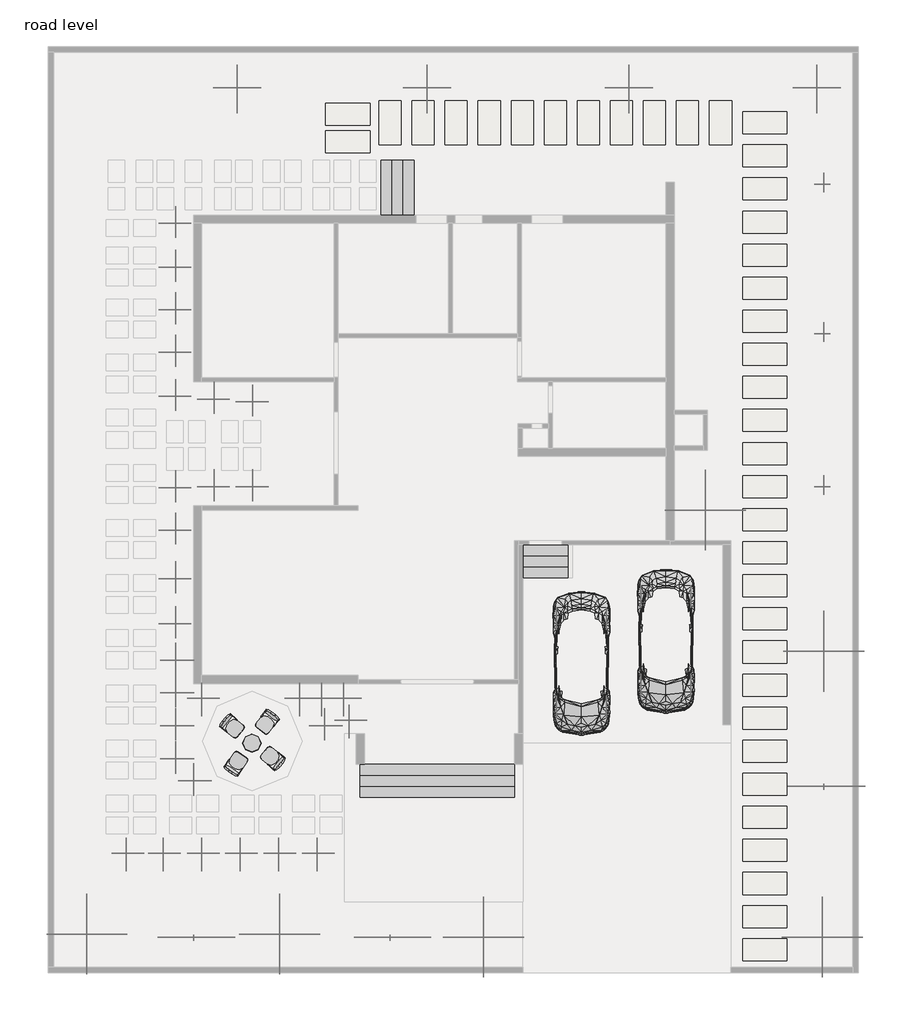
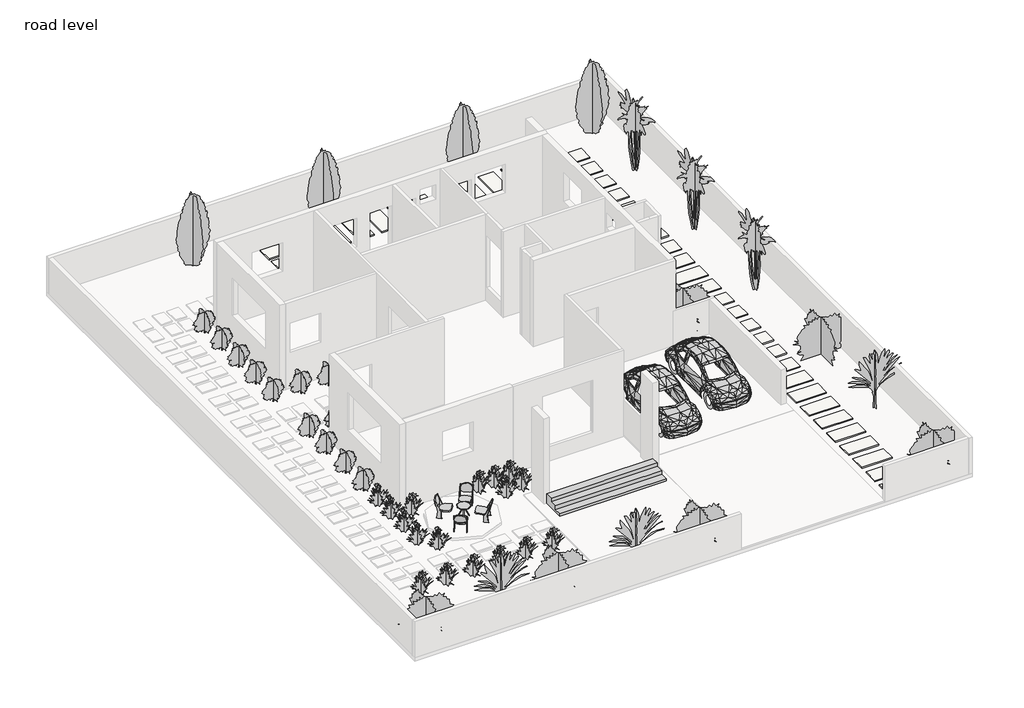
# One storey, part 3 of 3: 46 geographic elements, 8 furniture elements, 2 proxies, 1 slab.
"""IFC4 building model written with IfcOpenShell, lengths in millimetres."""

from ifc_helpers import new_model, si_unit, origin, origin_with_axes, place, context, project, spatial, polyline, outline, extrude, transform, mapped, element, save
from components import rpc_beetle_rpc_beetle_31f8b51e, casework_1_casework_1_95f3130b, casework_2_casework_2_cc4890fd, casework_3_casework_3_0f97de66, furniture_eb3a3c23, furniture_9d41381f, rpc_plant_tropical_55f6ff97, rpc_plant_tropical_jungle_flame_3_9c4808c2, rpc_shrub_d2795376, rpc_tree_deciduous_japanese_maple_10_8b15208c, rpc_tree_tropical_golden_malay_palm_10_e9996539, rpc_tree_tropical_japanese_fiber_banana_8_86d3d22d

model = new_model("IFC4")

# Units and contexts
model_context = context("Model", 3, world=origin())
ifc_project = project(units=[si_unit("LENGTHUNIT", "METRE", prefix="MILLI")], contexts=[model_context])

# Site, building, storey
site = spatial("IfcSite", under=ifc_project)
building = spatial("IfcBuilding", under=site)
storey = spatial("IfcBuildingStorey", under=building, Name="road level", Elevation=0.0)

# Proxies
placement = place(None, origin())
rpc_beetle_rpc_beetle_shape = rpc_beetle_rpc_beetle_31f8b51e(model_context)
element("IfcBuildingElementProxy", 1, Name="RPC Beetle : RPC Beetle", ObjectType="RPC Beetle : RPC Beetle", at=placement, inside=storey, context=model_context, shape_type="MappedRepresentation", body=[
    mapped(rpc_beetle_rpc_beetle_shape, transform((-917.8719122, 43.2168074, 50.8), x_axis=(-1.0, 0.0, 0.0), y_axis=(0.0, -1.0, 0.0), z_axis=(0.0, 0.0, 1.0))),
])
element("IfcBuildingElementProxy", 2, Name="RPC Beetle : RPC Beetle", ObjectType="RPC Beetle : RPC Beetle", at=placement, inside=storey, context=model_context, shape_type="MappedRepresentation", body=[
    mapped(rpc_beetle_rpc_beetle_shape, transform((-3254.6719122, -566.3831926, 50.8), x_axis=(-1.0, 0.0, 0.0), y_axis=(0.0, -1.0, 0.0), z_axis=(0.0, 0.0, 1.0))),
])

# Furniture
casework_1_casework_1_shape = casework_1_casework_1_95f3130b(model_context)
element("IfcFurniture", 3, ObjectType="Casework 1 : Casework 1", at=placement, inside=storey, context=model_context, shape_type="MappedRepresentation", body=[
    mapped(casework_1_casework_1_shape, transform((0.0, -844.55, -1397.3720703), x_axis=(1.0, 0.0, 0.0), y_axis=(0.0, 1.0, 0.0), z_axis=(0.0, 0.0, 1.0))),
])
casework_2_casework_2_shape = casework_2_casework_2_cc4890fd(model_context)
element("IfcFurniture", 4, ObjectType="Casework 2 : Casework 2", at=placement, inside=storey, context=model_context, shape_type="MappedRepresentation", body=[
    mapped(casework_2_casework_2_shape, transform((-2752.725, 0.0, -762.0), x_axis=(1.0, 0.0, 0.0), y_axis=(0.0, 1.0, 0.0), z_axis=(0.0, 0.0, 1.0))),
])
casework_3_casework_3_shape = casework_3_casework_3_0f97de66(model_context)
element("IfcFurniture", 5, ObjectType="Casework 3 : Casework 3", at=placement, inside=storey, context=model_context, shape_type="MappedRepresentation", body=[
    mapped(casework_3_casework_3_shape, transform((0.0, 5221.9554157, -2283.4751552), x_axis=(1.0, 0.0, 0.0), y_axis=(0.0, 1.0, 0.0), z_axis=(0.0, 0.0, 1.0))),
])
furniture_shape = furniture_eb3a3c23(model_context)
element("IfcFurniture", 6, ObjectType="Seating-Auditorium : 18\" x 24\" x 30\"", at=placement, inside=storey, context=model_context, shape_type="MappedRepresentation", body=[
    mapped(furniture_shape, transform((-12964.7044713, -3281.7150861, 152.4), x_axis=(-0.6438768453077839, -0.7651291447046678, 0.0), y_axis=(0.7651291447046678, -0.6438768453077839, 0.0), z_axis=(0.0, 0.0, 1.0))),
])
element("IfcFurniture", 7, ObjectType="Seating-Auditorium : 18\" x 24\" x 30\"", at=placement, inside=storey, context=model_context, shape_type="MappedRepresentation", body=[
    mapped(furniture_shape, transform((-11746.6183045, -4670.6974036, 152.4), x_axis=(0.6430165911827571, 0.7658522464964812, 0.0), y_axis=(-0.7658522464964812, 0.6430165911827571, 0.0), z_axis=(0.0, 0.0, 1.0))),
])
element("IfcFurniture", 8, ObjectType="Seating-Auditorium : 18\" x 24\" x 30\"", at=placement, inside=storey, context=model_context, shape_type="MappedRepresentation", body=[
    mapped(furniture_shape, transform((-11705.1193567, -3356.5011717, 152.4), x_axis=(-0.7919465740388523, 0.6105903895969252, 0.0), y_axis=(-0.6105903895969252, -0.7919465740388523, 0.0), z_axis=(0.0, 0.0, 1.0))),
])
element("IfcFurniture", 9, ObjectType="Seating-Auditorium : 18\" x 24\" x 30\"", at=placement, inside=storey, context=model_context, shape_type="MappedRepresentation", body=[
    mapped(furniture_shape, transform((-13054.2190924, -4639.820628, 152.4), x_axis=(0.8193621785920044, -0.5732762164026729, 0.0), y_axis=(0.5732762164026729, 0.8193621785920044, 0.0), z_axis=(0.0, 0.0, 1.0))),
])
furniture_2_shape = furniture_9d41381f(model_context)
element("IfcFurniture", 10, ObjectType="Table-Trio End : 20\" Diameter", at=placement, inside=storey, context=model_context, shape_type="MappedRepresentation", body=[
    mapped(furniture_2_shape, transform((-12373.2719122, -4001.7331926, 152.4), x_axis=(1.0, 0.0, 0.0), y_axis=(0.0, 1.0, 0.0), z_axis=(0.0, 0.0, 1.0))),
])

# Geographic elements
rpc_plant_tropical_shape = rpc_plant_tropical_55f6ff97(model_context)
element("IfcGeographicElement", 11, ObjectType="RPC Plant - Tropical", at=placement, inside=storey, context=model_context, shape_type="MappedRepresentation", body=[
    mapped(rpc_plant_tropical_shape, transform((-9833.2719122, -2757.1331926, 0.0), x_axis=(1.0, 0.0, 0.0), y_axis=(0.0, 1.0, 0.0), z_axis=(0.0, 0.0, 1.0))),
])
element("IfcGeographicElement", 12, ObjectType="RPC Plant - Tropical", at=placement, inside=storey, context=model_context, shape_type="MappedRepresentation", body=[
    mapped(rpc_plant_tropical_shape, transform((-9680.8719122, -3366.7331926, 0.0), x_axis=(1.0, 0.0, 0.0), y_axis=(0.0, 1.0, 0.0), z_axis=(0.0, 0.0, 1.0))),
])
element("IfcGeographicElement", 13, ObjectType="RPC Plant - Tropical", at=placement, inside=storey, context=model_context, shape_type="MappedRepresentation", body=[
    mapped(rpc_plant_tropical_shape, transform((-10442.8719122, -2757.1331926, 0.0), x_axis=(1.0, 0.0, 0.0), y_axis=(0.0, 1.0, 0.0), z_axis=(0.0, 0.0, 1.0))),
])
element("IfcGeographicElement", 14, ObjectType="RPC Plant - Tropical", at=placement, inside=storey, context=model_context, shape_type="MappedRepresentation", body=[
    mapped(rpc_plant_tropical_shape, transform((-11052.4719122, -2757.1331926, 0.0), x_axis=(1.0, 0.0, 0.0), y_axis=(0.0, 1.0, 0.0), z_axis=(0.0, 0.0, 1.0))),
])
element("IfcGeographicElement", 15, ObjectType="RPC Plant - Tropical", at=placement, inside=storey, context=model_context, shape_type="MappedRepresentation", body=[
    mapped(rpc_plant_tropical_shape, transform((-10366.6719122, -3519.1331926, 0.0), x_axis=(0.0, 1.0, 0.0), y_axis=(-1.0, 0.0, 0.0), z_axis=(0.0, 0.0, 1.0))),
])
element("IfcGeographicElement", 16, ObjectType="RPC Plant - Tropical", at=placement, inside=storey, context=model_context, shape_type="MappedRepresentation", body=[
    mapped(rpc_plant_tropical_shape, transform((-14481.4719122, -1709.3831926, 0.0), x_axis=(0.0, 1.0, 0.0), y_axis=(-1.0, 0.0, 0.0), z_axis=(0.0, 0.0, 1.0))),
])
element("IfcGeographicElement", 17, ObjectType="RPC Plant - Tropical", at=placement, inside=storey, context=model_context, shape_type="MappedRepresentation", body=[
    mapped(rpc_plant_tropical_shape, transform((-14481.4719122, -2604.7331926, 0.0), x_axis=(0.0, 1.0, 0.0), y_axis=(-1.0, 0.0, 0.0), z_axis=(0.0, 0.0, 1.0))),
])
element("IfcGeographicElement", 18, ObjectType="RPC Plant - Tropical", at=placement, inside=storey, context=model_context, shape_type="MappedRepresentation", body=[
    mapped(rpc_plant_tropical_shape, transform((-14481.4719122, -3519.1331926, 0.0), x_axis=(0.0, 1.0, 0.0), y_axis=(-1.0, 0.0, 0.0), z_axis=(0.0, 0.0, 1.0))),
])
element("IfcGeographicElement", 19, ObjectType="RPC Plant - Tropical", at=placement, inside=storey, context=model_context, shape_type="MappedRepresentation", body=[
    mapped(rpc_plant_tropical_shape, transform((-14481.4719122, -4433.5331926, 0.0), x_axis=(0.0, 1.0, 0.0), y_axis=(-1.0, 0.0, 0.0), z_axis=(0.0, 0.0, 1.0))),
])
element("IfcGeographicElement", 20, ObjectType="RPC Plant - Tropical", at=placement, inside=storey, context=model_context, shape_type="MappedRepresentation", body=[
    mapped(rpc_plant_tropical_shape, transform((-13986.1719122, -5043.1331926, 0.0), x_axis=(0.0, 1.0, 0.0), y_axis=(-1.0, 0.0, 0.0), z_axis=(0.0, 0.0, 1.0))),
])
element("IfcGeographicElement", 21, ObjectType="RPC Plant - Tropical", at=placement, inside=storey, context=model_context, shape_type="MappedRepresentation", body=[
    mapped(rpc_plant_tropical_shape, transform((-13757.5719122, -2757.1331926, 0.0), x_axis=(1.0, 0.0, 0.0), y_axis=(0.0, 1.0, 0.0), z_axis=(0.0, 0.0, 1.0))),
])
element("IfcGeographicElement", 22, ObjectType="RPC Plant - Tropical", at=placement, inside=storey, context=model_context, shape_type="MappedRepresentation", body=[
    mapped(rpc_plant_tropical_shape, transform((-15843.4576244, -7042.6627683, 0.0), x_axis=(1.0, 0.0, 0.0), y_axis=(0.0, 1.0, 0.0), z_axis=(0.0, 0.0, 1.0))),
])
element("IfcGeographicElement", 23, ObjectType="RPC Plant - Tropical", at=placement, inside=storey, context=model_context, shape_type="MappedRepresentation", body=[
    mapped(rpc_plant_tropical_shape, transform((-14827.4576244, -7042.6627683, 0.0), x_axis=(1.0, 0.0, 0.0), y_axis=(0.0, 1.0, 0.0), z_axis=(0.0, 0.0, 1.0))),
])
element("IfcGeographicElement", 24, ObjectType="RPC Plant - Tropical", at=placement, inside=storey, context=model_context, shape_type="MappedRepresentation", body=[
    mapped(rpc_plant_tropical_shape, transform((-13760.6576244, -7042.6627683, 0.0), x_axis=(1.0, 0.0, 0.0), y_axis=(0.0, 1.0, 0.0), z_axis=(0.0, 0.0, 1.0))),
])
element("IfcGeographicElement", 25, ObjectType="RPC Plant - Tropical", at=placement, inside=storey, context=model_context, shape_type="MappedRepresentation", body=[
    mapped(rpc_plant_tropical_shape, transform((-12703.4719122, -7042.6627683, 0.0), x_axis=(1.0, 0.0, 0.0), y_axis=(0.0, 1.0, 0.0), z_axis=(0.0, 0.0, 1.0))),
])
element("IfcGeographicElement", 26, ObjectType="RPC Plant - Tropical", at=placement, inside=storey, context=model_context, shape_type="MappedRepresentation", body=[
    mapped(rpc_plant_tropical_shape, transform((-11636.6719122, -7042.6627683, 0.0), x_axis=(1.0, 0.0, 0.0), y_axis=(0.0, 1.0, 0.0), z_axis=(0.0, 0.0, 1.0))),
])
element("IfcGeographicElement", 27, ObjectType="RPC Plant - Tropical", at=placement, inside=storey, context=model_context, shape_type="MappedRepresentation", body=[
    mapped(rpc_plant_tropical_shape, transform((-10569.8719122, -7042.6627683, 0.0), x_axis=(1.0, 0.0, 0.0), y_axis=(0.0, 1.0, 0.0), z_axis=(0.0, 0.0, 1.0))),
])
rpc_plant_tropical_jungle_flame_3_shape = rpc_plant_tropical_jungle_flame_3_9c4808c2(model_context)
element("IfcGeographicElement", 28, ObjectType="RPC Plant - Tropical : Jungle Flame - 3'", at=placement, inside=storey, context=model_context, shape_type="MappedRepresentation", body=[
    mapped(rpc_plant_tropical_jungle_flame_3_shape, transform((-12347.8719122, 3090.062262, 0.0), x_axis=(1.0, 0.0, 0.0), y_axis=(0.0, 1.0, 0.0), z_axis=(0.0, 0.0, 1.0))),
])
element("IfcGeographicElement", 29, ObjectType="RPC Plant - Tropical : Jungle Flame - 3'", at=placement, inside=storey, context=model_context, shape_type="MappedRepresentation", body=[
    mapped(rpc_plant_tropical_jungle_flame_3_shape, transform((-13414.6719122, 3090.062262, 0.0), x_axis=(1.0, 0.0, 0.0), y_axis=(0.0, 1.0, 0.0), z_axis=(0.0, 0.0, 1.0))),
])
element("IfcGeographicElement", 30, ObjectType="RPC Plant - Tropical : Jungle Flame - 3'", at=placement, inside=storey, context=model_context, shape_type="MappedRepresentation", body=[
    mapped(rpc_plant_tropical_jungle_flame_3_shape, transform((-14481.4719122, 3064.662262, 0.0), x_axis=(1.0, 0.0, 0.0), y_axis=(0.0, 1.0, 0.0), z_axis=(0.0, 0.0, 1.0))),
])
element("IfcGeographicElement", 31, ObjectType="RPC Plant - Tropical : Jungle Flame - 3'", at=placement, inside=storey, context=model_context, shape_type="MappedRepresentation", body=[
    mapped(rpc_plant_tropical_jungle_flame_3_shape, transform((-14481.4719122, 1891.0668074, 0.0), x_axis=(1.0, 0.0, 0.0), y_axis=(0.0, 1.0, 0.0), z_axis=(0.0, 0.0, 1.0))),
])
element("IfcGeographicElement", 32, ObjectType="RPC Plant - Tropical : Jungle Flame - 3'", at=placement, inside=storey, context=model_context, shape_type="MappedRepresentation", body=[
    mapped(rpc_plant_tropical_jungle_flame_3_shape, transform((-14481.4719122, 549.0309811, 0.0), x_axis=(1.0, 0.0, 0.0), y_axis=(0.0, 1.0, 0.0), z_axis=(0.0, 0.0, 1.0))),
])
element("IfcGeographicElement", 33, ObjectType="RPC Plant - Tropical : Jungle Flame - 3'", at=placement, inside=storey, context=model_context, shape_type="MappedRepresentation", body=[
    mapped(rpc_plant_tropical_jungle_flame_3_shape, transform((-14481.4719122, -699.7331926, 0.0), x_axis=(1.0, 0.0, 0.0), y_axis=(0.0, 1.0, 0.0), z_axis=(0.0, 0.0, 1.0))),
])
element("IfcGeographicElement", 34, ObjectType="RPC Plant - Tropical : Jungle Flame - 3'", at=placement, inside=storey, context=model_context, shape_type="MappedRepresentation", body=[
    mapped(rpc_plant_tropical_jungle_flame_3_shape, transform((-12347.8719122, 5434.3668074, 0.0), x_axis=(1.0, 0.0, 0.0), y_axis=(0.0, 1.0, 0.0), z_axis=(0.0, 0.0, 1.0))),
])
element("IfcGeographicElement", 35, ObjectType="RPC Plant - Tropical : Jungle Flame - 3'", at=placement, inside=storey, context=model_context, shape_type="MappedRepresentation", body=[
    mapped(rpc_plant_tropical_jungle_flame_3_shape, transform((-13414.6719122, 5510.5668074, 0.0), x_axis=(1.0, 0.0, 0.0), y_axis=(0.0, 1.0, 0.0), z_axis=(0.0, 0.0, 1.0))),
])
element("IfcGeographicElement", 36, ObjectType="RPC Plant - Tropical : Jungle Flame - 3'", at=placement, inside=storey, context=model_context, shape_type="MappedRepresentation", body=[
    mapped(rpc_plant_tropical_jungle_flame_3_shape, transform((-14481.4719122, 5586.7668074, 0.0), x_axis=(1.0, 0.0, 0.0), y_axis=(0.0, 1.0, 0.0), z_axis=(0.0, 0.0, 1.0))),
])
element("IfcGeographicElement", 37, ObjectType="RPC Plant - Tropical : Jungle Flame - 3'", at=placement, inside=storey, context=model_context, shape_type="MappedRepresentation", body=[
    mapped(rpc_plant_tropical_jungle_flame_3_shape, transform((-14481.4719122, 6805.9668074, 0.0), x_axis=(1.0, 0.0, 0.0), y_axis=(0.0, 1.0, 0.0), z_axis=(0.0, 0.0, 1.0))),
])
element("IfcGeographicElement", 38, ObjectType="RPC Plant - Tropical : Jungle Flame - 3'", at=placement, inside=storey, context=model_context, shape_type="MappedRepresentation", body=[
    mapped(rpc_plant_tropical_jungle_flame_3_shape, transform((-14481.4719122, 7983.8918074, 0.0), x_axis=(1.0, 0.0, 0.0), y_axis=(0.0, 1.0, 0.0), z_axis=(0.0, 0.0, 1.0))),
])
element("IfcGeographicElement", 39, ObjectType="RPC Plant - Tropical : Jungle Flame - 3'", at=placement, inside=storey, context=model_context, shape_type="MappedRepresentation", body=[
    mapped(rpc_plant_tropical_jungle_flame_3_shape, transform((-14481.4719122, 9161.8168074, 0.0), x_axis=(1.0, 0.0, 0.0), y_axis=(0.0, 1.0, 0.0), z_axis=(0.0, 0.0, 1.0))),
])
element("IfcGeographicElement", 40, ObjectType="RPC Plant - Tropical : Jungle Flame - 3'", at=placement, inside=storey, context=model_context, shape_type="MappedRepresentation", body=[
    mapped(rpc_plant_tropical_jungle_flame_3_shape, transform((-14481.4719122, 10368.3168074, 0.0), x_axis=(1.0, 0.0, 0.0), y_axis=(0.0, 1.0, 0.0), z_axis=(0.0, 0.0, 1.0))),
])
rpc_shrub_shape = rpc_shrub_d2795376(model_context)
element("IfcGeographicElement", 41, ObjectType="RPC Shrub", at=placement, inside=storey, context=model_context, shape_type="MappedRepresentation", body=[
    mapped(rpc_shrub_shape, transform((167.9780878, 2443.5168074, 0.0), x_axis=(1.0, 0.0, 0.0), y_axis=(0.0, 1.0, 0.0), z_axis=(0.0, 0.0, 1.0))),
])
element("IfcGeographicElement", 42, ObjectType="RPC Shrub", at=placement, inside=storey, context=model_context, shape_type="MappedRepresentation", body=[
    mapped(rpc_shrub_shape, transform((3447.8423756, -1464.9081926, 0.0), x_axis=(1.0, 0.0, 0.0), y_axis=(0.0, 1.0, 0.0), z_axis=(0.0, 0.0, 1.0))),
])
element("IfcGeographicElement", 43, ObjectType="RPC Shrub", at=placement, inside=storey, context=model_context, shape_type="MappedRepresentation", body=[
    mapped(rpc_shrub_shape, transform((3409.7423756, -9361.1331926, 0.0), x_axis=(1.0, 0.0, 0.0), y_axis=(0.0, 1.0, 0.0), z_axis=(0.0, 0.0, 1.0))),
])
element("IfcGeographicElement", 44, ObjectType="RPC Shrub", at=placement, inside=storey, context=model_context, shape_type="MappedRepresentation", body=[
    mapped(rpc_shrub_shape, transform((-16935.6576244, -9277.8627683, 0.0), x_axis=(1.0, 0.0, 0.0), y_axis=(0.0, 1.0, 0.0), z_axis=(0.0, 0.0, 1.0))),
])
element("IfcGeographicElement", 45, ObjectType="RPC Shrub", at=placement, inside=storey, context=model_context, shape_type="MappedRepresentation", body=[
    mapped(rpc_shrub_shape, transform((-11601.6576244, -9277.8627683, 0.0), x_axis=(1.0, 0.0, 0.0), y_axis=(0.0, 1.0, 0.0), z_axis=(0.0, 0.0, 1.0))),
])
element("IfcGeographicElement", 46, ObjectType="RPC Shrub", at=placement, inside=storey, context=model_context, shape_type="MappedRepresentation", body=[
    mapped(rpc_shrub_shape, transform((-5966.1219122, -9361.1331926, 0.0), x_axis=(1.0, 0.0, 0.0), y_axis=(0.0, 1.0, 0.0), z_axis=(0.0, 0.0, 1.0))),
])
rpc_tree_deciduous_japanese_maple_10_shape = rpc_tree_deciduous_japanese_maple_10_8b15208c(model_context)
element("IfcGeographicElement", 47, ObjectType="RPC Tree - Deciduous : Japanese Maple - 10'", at=placement, inside=storey, context=model_context, shape_type="MappedRepresentation", body=[
    mapped(rpc_tree_deciduous_japanese_maple_10_shape, transform((-7534.5719122, 14115.5372317, 0.0), x_axis=(1.0, 0.0, 0.0), y_axis=(0.0, 1.0, 0.0), z_axis=(0.0, 0.0, 1.0))),
])
element("IfcGeographicElement", 48, ObjectType="RPC Tree - Deciduous : Japanese Maple - 10'", at=placement, inside=storey, context=model_context, shape_type="MappedRepresentation", body=[
    mapped(rpc_tree_deciduous_japanese_maple_10_shape, transform((-12786.0219122, 14115.5372317, 0.0), x_axis=(1.0, 0.0, 0.0), y_axis=(0.0, 1.0, 0.0), z_axis=(0.0, 0.0, 1.0))),
])
element("IfcGeographicElement", 49, ObjectType="RPC Tree - Deciduous : Japanese Maple - 10'", at=placement, inside=storey, context=model_context, shape_type="MappedRepresentation", body=[
    mapped(rpc_tree_deciduous_japanese_maple_10_shape, transform((-1946.5719122, 14115.5372317, 0.0), x_axis=(1.0, 0.0, 0.0), y_axis=(0.0, 1.0, 0.0), z_axis=(0.0, 0.0, 1.0))),
])
element("IfcGeographicElement", 50, ObjectType="RPC Tree - Deciduous : Japanese Maple - 10'", at=placement, inside=storey, context=model_context, shape_type="MappedRepresentation", body=[
    mapped(rpc_tree_deciduous_japanese_maple_10_shape, transform((3257.3423756, 14115.5372317, 0.0), x_axis=(1.0, 0.0, 0.0), y_axis=(0.0, 1.0, 0.0), z_axis=(0.0, 0.0, 1.0))),
])
rpc_tree_tropical_golden_malay_palm_10_shape = rpc_tree_tropical_golden_malay_palm_10_e9996539(model_context)
element("IfcGeographicElement", 51, ObjectType="RPC Tree - Tropical : Golden Malay Palm - 10'", at=placement, inside=storey, context=model_context, shape_type="MappedRepresentation", body=[
    mapped(rpc_tree_tropical_golden_malay_palm_10_shape, transform((3447.8423756, 11448.5372317, 0.0), x_axis=(1.0, 0.0, 0.0), y_axis=(0.0, 1.0, 0.0), z_axis=(0.0, 0.0, 1.0))),
])
element("IfcGeographicElement", 52, ObjectType="RPC Tree - Tropical : Golden Malay Palm - 10'", at=placement, inside=storey, context=model_context, shape_type="MappedRepresentation", body=[
    mapped(rpc_tree_tropical_golden_malay_palm_10_shape, transform((3447.8423756, 7320.3168074, 0.0), x_axis=(1.0, 0.0, 0.0), y_axis=(0.0, 1.0, 0.0), z_axis=(0.0, 0.0, 1.0))),
])
element("IfcGeographicElement", 53, ObjectType="RPC Tree - Tropical : Golden Malay Palm - 10'", at=placement, inside=storey, context=model_context, shape_type="MappedRepresentation", body=[
    mapped(rpc_tree_tropical_golden_malay_palm_10_shape, transform((3447.8423756, 3090.062262, 0.0), x_axis=(1.0, 0.0, 0.0), y_axis=(0.0, 1.0, 0.0), z_axis=(0.0, 0.0, 1.0))),
])
rpc_tree_tropical_japanese_fiber_banana_8_shape = rpc_tree_tropical_japanese_fiber_banana_8_86d3d22d(model_context)
element("IfcGeographicElement", 54, ObjectType="RPC Tree - Tropical : Japanese Fiber Banana - 8'", at=placement, inside=storey, context=model_context, shape_type="MappedRepresentation", body=[
    mapped(rpc_tree_tropical_japanese_fiber_banana_8_shape, transform((3447.8423756, -5195.5331926, 0.0), x_axis=(1.0, 0.0, 0.0), y_axis=(0.0, 1.0, 0.0), z_axis=(0.0, 0.0, 1.0))),
])
element("IfcGeographicElement", 55, ObjectType="RPC Tree - Tropical : Japanese Fiber Banana - 8'", at=placement, inside=storey, context=model_context, shape_type="MappedRepresentation", body=[
    mapped(rpc_tree_tropical_japanese_fiber_banana_8_shape, transform((-13986.1719122, -9361.1331926, 0.0), x_axis=(1.0, 0.0, 0.0), y_axis=(0.0, 1.0, 0.0), z_axis=(0.0, 0.0, 1.0))),
])
element("IfcGeographicElement", 56, ObjectType="RPC Tree - Tropical : Japanese Fiber Banana - 8'", at=placement, inside=storey, context=model_context, shape_type="MappedRepresentation", body=[
    mapped(rpc_tree_tropical_japanese_fiber_banana_8_shape, transform((-8556.9219122, -9361.1331926, 0.0), x_axis=(1.0, 0.0, 0.0), y_axis=(0.0, 1.0, 0.0), z_axis=(0.0, 0.0, 1.0))),
])

# Slab
element("IfcSlab", 57, ObjectType="Generic - 2\" 6", at=placement, inside=storey, context=model_context, shape_type="SweptSolid", body=[
    extrude(outline(polyline([(2422.9605186, -10014.933976), (1203.7605186, -10014.933976), (1203.7605186, -9405.333976), (2422.9605186, -9405.333976), (2422.9605186, -10014.933976)])), origin_with_axes(), (0.0, 0.0, 1.0), 50.8),
    extrude(outline(polyline([(2422.9605186, -9100.533976), (1203.7605186, -9100.533976), (1203.7605186, -8490.933976), (2422.9605186, -8490.933976), (2422.9605186, -9100.533976)])), origin_with_axes(), (0.0, 0.0, 1.0), 50.8),
    extrude(outline(polyline([(2422.9605186, -8186.133976), (1203.7605186, -8186.133976), (1203.7605186, -7576.533976), (2422.9605186, -7576.533976), (2422.9605186, -8186.133976)])), origin_with_axes(), (0.0, 0.0, 1.0), 50.8),
    extrude(outline(polyline([(2422.9605186, -7271.733976), (1203.7605186, -7271.733976), (1203.7605186, -6662.133976), (2422.9605186, -6662.133976), (2422.9605186, -7271.733976)])), origin_with_axes(), (0.0, 0.0, 1.0), 50.8),
    extrude(outline(polyline([(2422.9605186, -6357.333976), (1203.7605186, -6357.333976), (1203.7605186, -5747.733976), (2422.9605186, -5747.733976), (2422.9605186, -6357.333976)])), origin_with_axes(), (0.0, 0.0, 1.0), 50.8),
    extrude(outline(polyline([(2422.9605186, -5442.933976), (1203.7605186, -5442.933976), (1203.7605186, -4833.333976), (2422.9605186, -4833.333976), (2422.9605186, -5442.933976)])), origin_with_axes(), (0.0, 0.0, 1.0), 50.8),
    extrude(outline(polyline([(2422.9605186, -4528.533976), (1203.7605186, -4528.533976), (1203.7605186, -3918.933976), (2422.9605186, -3918.933976), (2422.9605186, -4528.533976)])), origin_with_axes(), (0.0, 0.0, 1.0), 50.8),
    extrude(outline(polyline([(2422.9605186, -3614.133976), (1203.7605186, -3614.133976), (1203.7605186, -3004.533976), (2422.9605186, -3004.533976), (2422.9605186, -3614.133976)])), origin_with_axes(), (0.0, 0.0, 1.0), 50.8),
    extrude(outline(polyline([(2422.9605186, -2699.733976), (1203.7605186, -2699.733976), (1203.7605186, -2090.133976), (2422.9605186, -2090.133976), (2422.9605186, -2699.733976)])), origin_with_axes(), (0.0, 0.0, 1.0), 50.8),
    extrude(outline(polyline([(2422.9605186, -1785.333976), (1203.7605186, -1785.333976), (1203.7605186, -1175.733976), (2422.9605186, -1175.733976), (2422.9605186, -1785.333976)])), origin_with_axes(), (0.0, 0.0, 1.0), 50.8),
    extrude(outline(polyline([(2422.9605186, -870.933976), (1203.7605186, -870.933976), (1203.7605186, -261.333976), (2422.9605186, -261.333976), (2422.9605186, -870.933976)])), origin_with_axes(), (0.0, 0.0, 1.0), 50.8),
    extrude(outline(polyline([(2422.9605186, 43.466024), (1203.7605186, 43.466024), (1203.7605186, 653.066024), (2422.9605186, 653.066024), (2422.9605186, 43.466024)])), origin_with_axes(), (0.0, 0.0, 1.0), 50.8),
    extrude(outline(polyline([(2422.9605186, 957.866024), (1203.7605186, 957.866024), (1203.7605186, 1567.466024), (2422.9605186, 1567.466024), (2422.9605186, 957.866024)])), origin_with_axes(), (0.0, 0.0, 1.0), 50.8),
    extrude(outline(polyline([(2422.9605186, 1872.266024), (1203.7605186, 1872.266024), (1203.7605186, 2481.866024), (2422.9605186, 2481.866024), (2422.9605186, 1872.266024)])), origin_with_axes(), (0.0, 0.0, 1.0), 50.8),
    extrude(outline(polyline([(2422.9605186, 2786.666024), (1203.7605186, 2786.666024), (1203.7605186, 3396.266024), (2422.9605186, 3396.266024), (2422.9605186, 2786.666024)])), origin_with_axes(), (0.0, 0.0, 1.0), 50.8),
    extrude(outline(polyline([(2422.9605186, 3701.066024), (1203.7605186, 3701.066024), (1203.7605186, 4310.666024), (2422.9605186, 4310.666024), (2422.9605186, 3701.066024)])), origin_with_axes(), (0.0, 0.0, 1.0), 50.8),
    extrude(outline(polyline([(2422.9605186, 4615.466024), (1203.7605186, 4615.466024), (1203.7605186, 5225.066024), (2422.9605186, 5225.066024), (2422.9605186, 4615.466024)])), origin_with_axes(), (0.0, 0.0, 1.0), 50.8),
    extrude(outline(polyline([(2422.9605186, 5529.866024), (1203.7605186, 5529.866024), (1203.7605186, 6139.466024), (2422.9605186, 6139.466024), (2422.9605186, 5529.866024)])), origin_with_axes(), (0.0, 0.0, 1.0), 50.8),
    extrude(outline(polyline([(2422.9605186, 6444.266024), (1203.7605186, 6444.266024), (1203.7605186, 7053.866024), (2422.9605186, 7053.866024), (2422.9605186, 6444.266024)])), origin_with_axes(), (0.0, 0.0, 1.0), 50.8),
    extrude(outline(polyline([(2422.9605186, 7358.666024), (1203.7605186, 7358.666024), (1203.7605186, 7968.266024), (2422.9605186, 7968.266024), (2422.9605186, 7358.666024)])), origin_with_axes(), (0.0, 0.0, 1.0), 50.8),
    extrude(outline(polyline([(2422.9605186, 8273.066024), (1203.7605186, 8273.066024), (1203.7605186, 8882.666024), (2422.9605186, 8882.666024), (2422.9605186, 8273.066024)])), origin_with_axes(), (0.0, 0.0, 1.0), 50.8),
    extrude(outline(polyline([(2422.9605186, 9187.466024), (1203.7605186, 9187.466024), (1203.7605186, 9797.066024), (2422.9605186, 9797.066024), (2422.9605186, 9187.466024)])), origin_with_axes(), (0.0, 0.0, 1.0), 50.8),
    extrude(outline(polyline([(2422.9605186, 10101.866024), (1203.7605186, 10101.866024), (1203.7605186, 10711.466024), (2422.9605186, 10711.466024), (2422.9605186, 10101.866024)])), origin_with_axes(), (0.0, 0.0, 1.0), 50.8),
    extrude(outline(polyline([(2422.9605186, 11016.266024), (1203.7605186, 11016.266024), (1203.7605186, 11625.866024), (2422.9605186, 11625.866024), (2422.9605186, 11016.266024)])), origin_with_axes(), (0.0, 0.0, 1.0), 50.8),
    extrude(outline(polyline([(2422.9605186, 11930.666024), (1203.7605186, 11930.666024), (1203.7605186, 12540.266024), (2422.9605186, 12540.266024), (2422.9605186, 11930.666024)])), origin_with_axes(), (0.0, 0.0, 1.0), 50.8),
    extrude(outline(polyline([(2422.9605186, 12845.066024), (1203.7605186, 12845.066024), (1203.7605186, 13454.666024), (2422.9605186, 13454.666024), (2422.9605186, 12845.066024)])), origin_with_axes(), (0.0, 0.0, 1.0), 50.8),
    extrude(outline(polyline([(898.9605186, 13759.466024), (898.9605186, 12540.266024), (289.3605186, 12540.266024), (289.3605186, 13759.466024), (898.9605186, 13759.466024)])), origin_with_axes(), (0.0, 0.0, 1.0), 50.8),
    extrude(outline(polyline([(-15.4394814, 13759.466024), (-15.4394814, 12540.266024), (-625.0394814, 12540.266024), (-625.0394814, 13759.466024), (-15.4394814, 13759.466024)])), origin_with_axes(), (0.0, 0.0, 1.0), 50.8),
    extrude(outline(polyline([(-929.8394814, 13759.466024), (-929.8394814, 12540.266024), (-1539.4394814, 12540.266024), (-1539.4394814, 13759.466024), (-929.8394814, 13759.466024)])), origin_with_axes(), (0.0, 0.0, 1.0), 50.8),
    extrude(outline(polyline([(-1844.2394814, 13759.466024), (-1844.2394814, 12540.266024), (-2453.8394814, 12540.266024), (-2453.8394814, 13759.466024), (-1844.2394814, 13759.466024)])), origin_with_axes(), (0.0, 0.0, 1.0), 50.8),
    extrude(outline(polyline([(-2758.6394814, 13759.466024), (-2758.6394814, 12540.266024), (-3368.2394814, 12540.266024), (-3368.2394814, 13759.466024), (-2758.6394814, 13759.466024)])), origin_with_axes(), (0.0, 0.0, 1.0), 50.8),
    extrude(outline(polyline([(-3673.0394814, 13759.466024), (-3673.0394814, 12540.266024), (-4282.6394814, 12540.266024), (-4282.6394814, 13759.466024), (-3673.0394814, 13759.466024)])), origin_with_axes(), (0.0, 0.0, 1.0), 50.8),
    extrude(outline(polyline([(-4587.4394814, 13759.466024), (-4587.4394814, 12540.266024), (-5197.0394814, 12540.266024), (-5197.0394814, 13759.466024), (-4587.4394814, 13759.466024)])), origin_with_axes(), (0.0, 0.0, 1.0), 50.8),
    extrude(outline(polyline([(-5501.8394814, 13759.466024), (-5501.8394814, 12540.266024), (-6111.4394814, 12540.266024), (-6111.4394814, 13759.466024), (-5501.8394814, 13759.466024)])), origin_with_axes(), (0.0, 0.0, 1.0), 50.8),
    extrude(outline(polyline([(-6416.2394814, 13759.466024), (-6416.2394814, 12540.266024), (-7025.8394814, 12540.266024), (-7025.8394814, 13759.466024), (-6416.2394814, 13759.466024)])), origin_with_axes(), (0.0, 0.0, 1.0), 50.8),
    extrude(outline(polyline([(-7330.6394814, 13759.466024), (-7330.6394814, 12540.266024), (-7940.2394814, 12540.266024), (-7940.2394814, 13759.466024), (-7330.6394814, 13759.466024)])), origin_with_axes(), (0.0, 0.0, 1.0), 50.8),
    extrude(outline(polyline([(-8245.0394814, 13759.466024), (-8245.0394814, 12540.266024), (-8854.6394814, 12540.266024), (-8854.6394814, 13759.466024), (-8245.0394814, 13759.466024)])), origin_with_axes(), (0.0, 0.0, 1.0), 50.8),
    extrude(outline(polyline([(-9108.6394814, 12318.016024), (-10327.8394814, 12318.016024), (-10327.8394814, 12927.616024), (-9108.6394814, 12927.616024), (-9108.6394814, 12318.016024)])), origin_with_axes(), (0.0, 0.0, 1.0), 50.8),
    extrude(outline(polyline([(-9108.6394814, 13080.016024), (-10327.8394814, 13080.016024), (-10327.8394814, 13689.616024), (-9108.6394814, 13689.616024), (-9108.6394814, 13080.016024)])), origin_with_axes(), (0.0, 0.0, 1.0), 50.8),
])

save(model, "model.ifc")

# Revit data of these elements
# Type "RPC Beetle : RPC Beetle"
#   built-in parameter 1005198 = "{2, 15},{39, RPC-16-0U6E-L4EG-ENH1-J3KF-SVEL-0TX4-C0},{1, 0},{1, 0},{2, 34},{2, 11},{20, AdvancedUIDefinition},{1, 0},{1, 0},{0, },{2, 11},{10, AssetLibID},{1, 0},{1, 0},{36, 4D3F6E72-3F99-4203-98E9-AF80B3C7A7A4},{2, 11},{10, BaseSchema},{1, 0},{1, 0},{9, RPCSchema},{2, 11},{12, ExchangeGUID},{1, 0},{1, 0},{0, },{1, 2},{6, Hidden},{1, 0},{1, 0},{1, 0},{2, 11},{12, LocalizedUID},{1, 0},{1, 0},{0, },{1, 4},{11, RPCCategory},{1, 0},{1, 0},{1, 0},{2, 11},{11, RPCFilePath},{1, 0},{1, 0},{115, C:\\Program Files\\Common Files\\Autodesk Shared\\Materials\\4\\assetlibrary_base.fbm\\RPCs\\ArchVision_Demo_VW_Beetle4.rpc},{2, 11},{8, RPCImage},{1, 0},{1, 0},{0, },{1, 6},{14, RPCPlantHeight},{1, 0},{1, 0},{1, 0},{2, 11},{9, RPCTypeId},{1, 0},{1, 0},{39, RPC-16-0U6E-L4EG-ENH1-J3KF-SVEL-0TX4-C0},{1, 4},{13, SchemaVersion},{1, 0},{1, 0},{1, 5},{2, 11},{12, UIDefinition},{1, 0},{1, 0},{0, },{2, 11},{6, UIName},{1, 0},{1, 0},{39, RPC-16-0U6E-L4EG-ENH1-J3KF-SVEL-0TX4-C0},{2, 11},{11, VersionGUID},{1, 0},{1, 0},{9, RPCSchema},{2, 11},{9, assettype},{1, 0},{1, 0},{11, RPCGeometry},{2, 11},{8, category},{1, 0},{1, 0},{21, :Auto_Economy/Midsize},{2, 11},{11, description},{1, 0},{1, 0},{0, },{2, 11},{7, keyword},{1, 0},{1, 0},{27, :Geometry:RPC:VW Beetle [4]},{2, 11},{9, localname},{1, 0},{1, 0},{3, RPC},{2, 11},{9, localtype},{1, 0},{1, 0},{3, RPC},{1, 4},{8, revision},{1, 0},{1, 0},{1, 1},{2, 11},{9, thumbnail},{1, 0},{1, 0},{0, },{1, 4},{7, version},{1, 0},{1, 0},{1, 1},{2, 14},{6, Height},{1, 0},{1, 0},{7, 4.91667},{1, 2},{20, RPC_Cast Reflections},{1, 0},{1, 0},{1, 1},{1, 4},{16, RPC_Transparency},{1, 0},{1, 0},{2, 14},{1, 4},{11, RPC_Tinting},{1, 0},{1, 0},{2, 44},{1, 2},{15, RPC_Use Tinting},{1, 0},{1, 0},{1, 0},{1, 2},{17, RPC_License Plate},{1, 0},{1, 0},{1, 0},{2, 11},{25, RPC_License Plate Texture},{1, 0},{1, 0},{64, __RPC:/object data/textures/car/plate/textures/default/rgb/0/0/0},{2, 11},{27, RPC_i_License Plate Texture},{1, 0},{1, 0},{0, },{1, 2},{16, RPC_Custom Plate},{1, 0},{1, 0},{1, 0},{2, 11},{27, RPC_License Plate File Name},{1, 0},{1, 0},{0, },{21, assetlibrary_base.fbx},{1, 5},"
#   built-in parameter 1005195 = "RPC-16-0U6E-L4EG-ENH1-J3KF-SVEL-0TX4-C0"
#   Height = 0
# Type "Seating-Auditorium : 18\" x 24\" x 30\""
#   Assembly Code = "E2020200"
#   Seat Material = Linen, Beige
#   Frame Material = Steel, Paint Finish, Dark Gray, Matte
#   Default Elevation = 0
# Type "Table-Trio End : 20\" Diameter"
#   Assembly Code = "E2020200"
#   Default Elevation = 0' - 6"
#   Base and Trim Material = Wood - Birch
#   Table Top Material = Laminate - Ivory,Matte
# Type "RPC Plant - Tropical"
#   built-in parameter 1005198 = "{2, 15},{39, RPC-16-FWM5-GM7X-C67P-4000-ST1L-LVER-AU},{1, 0},{1, 0},{2, 35},{1, 8},{5, Color},{1, 0},{1, 0},{3, 0.8},{3, 0.8},{3, 0.8},{1, 8},{7, BBoxMin},{1, 0},{1, 0},{1, 0},{1, 0},{1, 0},{1, 8},{7, BBoxMax},{1, 0},{1, 0},{1, 0},{1, 0},{1, 0},{2, 11},{9, RPCTypeId},{1, 0},{1, 0},{39, RPC-16-FWM5-GM7X-C67P-4000-ST1L-LVER-AU},{1, 6},{14, RPCPlantHeight},{1, 0},{1, 0},{1, 3},{2, 11},{7, keyword},{1, 0},{1, 0},{99, :Geometry:RPC:Crane Lily:strelitzia:reinae:crane lily:plants:shrub:flower:tropical:bird-of-paradise},{2, 11},{8, category},{1, 0},{1, 0},{17, :Shrubs [General]},{2, 11},{12, LocalizedUID},{1, 0},{1, 0},{10, Crane Lily},{2, 14},{6, Height},{1, 0},{1, 0},{1, 3},{1, 2},{16, Cast Reflections},{1, 0},{1, 0},{1, 0},{1, 2},{12, Cast Shadows},{1, 0},{1, 0},{1, 1},{1, 2},{9, Lock View},{1, 0},{1, 0},{1, 0},{1, 4},{5, ViewC},{1, 0},{1, 0},{1, 0},{2, 11},{20, AdvancedUIDefinition},{1, 0},{1, 0},{0, },{2, 11},{10, AssetLibID},{1, 0},{1, 0},{36, 4D3F6E72-3F99-4203-98E9-AF80B3C7A7A4},{2, 11},{10, BaseSchema},{1, 0},{1, 0},{9, RPCSchema},{2, 11},{12, ExchangeGUID},{1, 0},{1, 0},{0, },{1, 2},{6, Hidden},{1, 0},{1, 0},{1, 0},{1, 4},{11, RPCCategory},{1, 0},{1, 0},{1, 0},{2, 11},{8, RPCImage},{1, 0},{1, 0},{0, },{1, 4},{13, SchemaVersion},{1, 0},{1, 0},{1, 4},{2, 11},{12, UIDefinition},{1, 0},{1, 0},{0, },{2, 11},{6, UIName},{1, 0},{1, 0},{39, RPC-16-FWM5-GM7X-C67P-4000-ST1L-LVER-AU},{2, 11},{11, VersionGUID},{1, 0},{1, 0},{9, RPCSchema},{2, 11},{9, assettype},{1, 0},{1, 0},{11, RPCGeometry},{2, 11},{11, description},{1, 0},{1, 0},{0, },{2, 11},{9, localname},{1, 0},{1, 0},{3, RPC},{2, 11},{9, localtype},{1, 0},{1, 0},{3, RPC},{1, 4},{8, revision},{1, 0},{1, 0},{1, 1},{2, 11},{9, thumbnail},{1, 0},{1, 0},{0, },{1, 4},{7, version},{1, 0},{1, 0},{1, 1},{1, 2},{20, RPC_Cast Reflections},{1, 0},{1, 0},{1, 1},{1, 2},{16, RPC_Cast Shadows},{1, 0},{1, 0},{1, 1},{1, 2},{13, RPC_Lock View},{1, 0},{1, 0},{1, 0},{1, 4},{9, RPC_ViewC},{1, 0},{1, 0},{1, 0},{21, assetlibrary_base.fbx},{1, 5},"
#   built-in parameter 1005195 = "RPC-16-FWM5-GM7X-C67P-4000-ST1L-LVER-AU"
#   Assembly Code = "G2050500"
#   Height = 3' - 0"
#   Default Elevation = 0
# Type "RPC Plant - Tropical : Jungle Flame - 3'"
#   built-in parameter 1005198 = "{2, 15},{39, RPC-16-FUVJ-JWG0-MWGK-8000-ST1L-LVER-AU},{1, 0},{1, 0},{2, 35},{1, 8},{5, Color},{1, 0},{1, 0},{3, 0.8},{3, 0.8},{3, 0.8},{1, 8},{7, BBoxMin},{1, 0},{1, 0},{1, 0},{1, 0},{1, 0},{1, 8},{7, BBoxMax},{1, 0},{1, 0},{1, 0},{1, 0},{1, 0},{2, 11},{9, RPCTypeId},{1, 0},{1, 0},{39, RPC-16-FUVJ-JWG0-MWGK-8000-ST1L-LVER-AU},{1, 6},{14, RPCPlantHeight},{1, 0},{1, 0},{1, 3},{2, 11},{7, keyword},{1, 0},{1, 0},{90, :Geometry:RPC:Jungle Flame:ixora macrothyrsa:jungle flame:bush:shrub:plant:flower:tropical},{2, 11},{8, category},{1, 0},{1, 0},{17, :Shrubs [General]},{2, 11},{12, LocalizedUID},{1, 0},{1, 0},{12, Jungle Flame},{2, 14},{6, Height},{1, 0},{1, 0},{1, 3},{1, 2},{16, Cast Reflections},{1, 0},{1, 0},{1, 0},{1, 2},{12, Cast Shadows},{1, 0},{1, 0},{1, 1},{1, 2},{9, Lock View},{1, 0},{1, 0},{1, 0},{1, 4},{5, ViewC},{1, 0},{1, 0},{1, 0},{2, 11},{20, AdvancedUIDefinition},{1, 0},{1, 0},{0, },{2, 11},{10, AssetLibID},{1, 0},{1, 0},{36, 4D3F6E72-3F99-4203-98E9-AF80B3C7A7A4},{2, 11},{10, BaseSchema},{1, 0},{1, 0},{9, RPCSchema},{2, 11},{12, ExchangeGUID},{1, 0},{1, 0},{0, },{1, 2},{6, Hidden},{1, 0},{1, 0},{1, 0},{1, 4},{11, RPCCategory},{1, 0},{1, 0},{1, 0},{2, 11},{8, RPCImage},{1, 0},{1, 0},{0, },{1, 4},{13, SchemaVersion},{1, 0},{1, 0},{1, 4},{2, 11},{12, UIDefinition},{1, 0},{1, 0},{0, },{2, 11},{6, UIName},{1, 0},{1, 0},{39, RPC-16-FUVJ-JWG0-MWGK-8000-ST1L-LVER-AU},{2, 11},{11, VersionGUID},{1, 0},{1, 0},{9, RPCSchema},{2, 11},{9, assettype},{1, 0},{1, 0},{11, RPCGeometry},{2, 11},{11, description},{1, 0},{1, 0},{0, },{2, 11},{9, localname},{1, 0},{1, 0},{3, RPC},{2, 11},{9, localtype},{1, 0},{1, 0},{3, RPC},{1, 4},{8, revision},{1, 0},{1, 0},{1, 1},{2, 11},{9, thumbnail},{1, 0},{1, 0},{0, },{1, 4},{7, version},{1, 0},{1, 0},{1, 1},{1, 2},{20, RPC_Cast Reflections},{1, 0},{1, 0},{1, 1},{1, 2},{16, RPC_Cast Shadows},{1, 0},{1, 0},{1, 1},{1, 2},{13, RPC_Lock View},{1, 0},{1, 0},{1, 0},{1, 4},{9, RPC_ViewC},{1, 0},{1, 0},{1, 0},{21, assetlibrary_base.fbx},{1, 5},"
#   built-in parameter 1005195 = "RPC-16-FUVJ-JWG0-MWGK-8000-ST1L-LVER-AU"
#   Type Comments = "Jungle Flame"
#   Assembly Code = "G2050500"
#   Height = 3' - 0"
#   Default Elevation = 0
# Type "RPC Shrub"
#   built-in parameter 1005198 = "{2, 15},{39, RPC-16-G3GJ-A6PX-PK1P-U000-ST1L-LVER-AU},{1, 0},{1, 0},{2, 35},{1, 8},{5, Color},{1, 0},{1, 0},{3, 0.8},{3, 0.8},{3, 0.8},{1, 8},{7, BBoxMin},{1, 0},{1, 0},{1, 0},{1, 0},{1, 0},{1, 8},{7, BBoxMax},{1, 0},{1, 0},{1, 0},{1, 0},{1, 0},{2, 11},{9, RPCTypeId},{1, 0},{1, 0},{39, RPC-16-G3GJ-A6PX-PK1P-U000-ST1L-LVER-AU},{1, 6},{14, RPCPlantHeight},{1, 0},{1, 0},{7, 5.33333},{2, 11},{7, keyword},{1, 0},{1, 0},{22, :Geometry:RPC:Oleander},{2, 11},{8, category},{1, 0},{1, 0},{17, :Shrubs & Grasses},{2, 11},{12, LocalizedUID},{1, 0},{1, 0},{8, Oleander},{2, 14},{6, Height},{1, 0},{1, 0},{7, 5.33333},{1, 2},{16, Cast Reflections},{1, 0},{1, 0},{1, 0},{1, 2},{12, Cast Shadows},{1, 0},{1, 0},{1, 1},{1, 2},{9, Lock View},{1, 0},{1, 0},{1, 0},{1, 4},{5, ViewC},{1, 0},{1, 0},{1, 0},{2, 11},{20, AdvancedUIDefinition},{1, 0},{1, 0},{0, },{2, 11},{10, AssetLibID},{1, 0},{1, 0},{36, 4D3F6E72-3F99-4203-98E9-AF80B3C7A7A4},{2, 11},{10, BaseSchema},{1, 0},{1, 0},{9, RPCSchema},{2, 11},{12, ExchangeGUID},{1, 0},{1, 0},{0, },{1, 2},{6, Hidden},{1, 0},{1, 0},{1, 0},{1, 4},{11, RPCCategory},{1, 0},{1, 0},{1, 0},{2, 11},{8, RPCImage},{1, 0},{1, 0},{0, },{1, 4},{13, SchemaVersion},{1, 0},{1, 0},{1, 4},{2, 11},{12, UIDefinition},{1, 0},{1, 0},{0, },{2, 11},{6, UIName},{1, 0},{1, 0},{39, RPC-16-G3GJ-A6PX-PK1P-U000-ST1L-LVER-AU},{2, 11},{11, VersionGUID},{1, 0},{1, 0},{9, RPCSchema},{2, 11},{9, assettype},{1, 0},{1, 0},{11, RPCGeometry},{2, 11},{11, description},{1, 0},{1, 0},{0, },{2, 11},{9, localname},{1, 0},{1, 0},{3, RPC},{2, 11},{9, localtype},{1, 0},{1, 0},{3, RPC},{1, 4},{8, revision},{1, 0},{1, 0},{1, 1},{2, 11},{9, thumbnail},{1, 0},{1, 0},{0, },{1, 4},{7, version},{1, 0},{1, 0},{1, 1},{1, 2},{20, RPC_Cast Reflections},{1, 0},{1, 0},{1, 1},{1, 2},{16, RPC_Cast Shadows},{1, 0},{1, 0},{1, 1},{1, 2},{13, RPC_Lock View},{1, 0},{1, 0},{1, 0},{1, 4},{9, RPC_ViewC},{1, 0},{1, 0},{1, 0},{21, assetlibrary_base.fbx},{1, 5},"
#   built-in parameter 1005195 = "RPC-16-G3GJ-A6PX-PK1P-U000-ST1L-LVER-AU"
#   Assembly Code = "G2050500"
#   Height = 5' - 4"
#   Default Elevation = 0
# Type "RPC Tree - Deciduous : Japanese Maple - 10'"
#   built-in parameter 1005195 = "RPC-16-FUM3-UUQ0-UBF0-N000-ST1L-LVER-AU"
#   Type Comments = "Japanese Maple"
#   Assembly Code = "G2050500"
#   Height = 10' - 0"
#   Default Elevation = 0
# Type "RPC Tree - Tropical : Golden Malay Palm - 10'"
#   built-in parameter 1005195 = "RPC-16-FXGL-UL7X-PH44-0000-ST1L-LVER-AU"
#   Type Comments = "Golden Malay Palm"
#   Assembly Code = "G2050500"
#   Height = 10' - 0"
#   Plan Symbol = element 497571
#   Default Elevation = 0
# Type "RPC Tree - Tropical : Japanese Fiber Banana - 8'"
#   built-in parameter 1005195 = "RPC-16-G2M6-EAFX-C5H6-W000-ST1L-LVER-AU"
#   Type Comments = "Japanese Fiber Banana"
#   Assembly Code = "G2050500"
#   Height = 8' - 0"
#   Plan Symbol = element 497571
#   Default Elevation = 0
# Type "Generic - 2\" 6"
#   Assembly Code = "B1010"
#   Function = 0
#   Layers, outside or top first: 0' - 2" "Tile, Porcelain, 4in" (function 1)
# Elements 1, 2 (IfcBuildingElementProxy, "RPC Beetle : RPC Beetle")
#   Phase Created = New Construction
# Element 3 (IfcFurniture, "Casework 1 : Casework 1")
#   Phase Created = New Construction
# Element 4 (IfcFurniture, "Casework 2 : Casework 2")
#   Phase Created = New Construction
# Element 5 (IfcFurniture, "Casework 3 : Casework 3")
#   Phase Created = New Construction
# Elements 6, 7, 8, 9 (IfcFurniture, "Seating-Auditorium : 18\" x 24\" x 30\"")
#   Phase Created = New Construction
#   Materials on its faces: "Steel, Paint Finish, Dark Gray, Matte", "Linen, Beige"
# Element 10 (IfcFurniture, "Table-Trio End : 20\" Diameter")
#   Phase Created = New Construction
#   Materials on its faces: "Wood - Birch", "Laminate - Ivory,Matte"
# Elements 11, 12, 13, 14, 15, 16, 17, 18, 19, 20, 21, 22, 23, 24, 25, 26, 27 (IfcGeographicElement, "RPC Plant - Tropical")
#   Phase Created = New Construction
# Elements 28, 29, 30, 31, 32, 33, 34, 35, 36, 37, 38, 39, 40 (IfcGeographicElement, "RPC Plant - Tropical : Jungle Flame - 3'")
#   Phase Created = New Construction
# Elements 41, 42, 43, 44, 45, 46 (IfcGeographicElement, "RPC Shrub")
#   Phase Created = New Construction
# Elements 47, 48, 49, 50 (IfcGeographicElement, "RPC Tree - Deciduous : Japanese Maple - 10'")
#   Phase Created = New Construction
# Elements 51, 52, 53 (IfcGeographicElement, "RPC Tree - Tropical : Golden Malay Palm - 10'")
#   Phase Created = New Construction
# Elements 54, 55, 56 (IfcGeographicElement, "RPC Tree - Tropical : Japanese Fiber Banana - 8'")
#   Phase Created = New Construction
# Element 57 (IfcSlab, "Generic - 2\" 6")
#   Height Offset From Level = 0' - 2"
#   Phase Created = New Construction
#   Materials on its faces: "Tile, Porcelain, 4in"
# Materials
#   "Linen, Beige": class "Textile", colour RGB 249 239 230, transparency 0, Description = "Linen, beige", Cost = 0
#   "Steel, Paint Finish, Dark Gray, Matte": class "Metal", colour RGB 0 0 0, transparency 0, Description = "Steel, paint finish, dark gray, matte", Cost = 0
#   "Wood - Birch": colour RGB 230 196 162, transparency 0
#   "Laminate - Ivory,Matte": colour RGB 127 127 127, transparency 0
#   "Tile, Porcelain, 4in": class "Generic", colour RGB 89 87 158, transparency 0, Description = "Porcelain tile, 4\", white", Cost = 0
